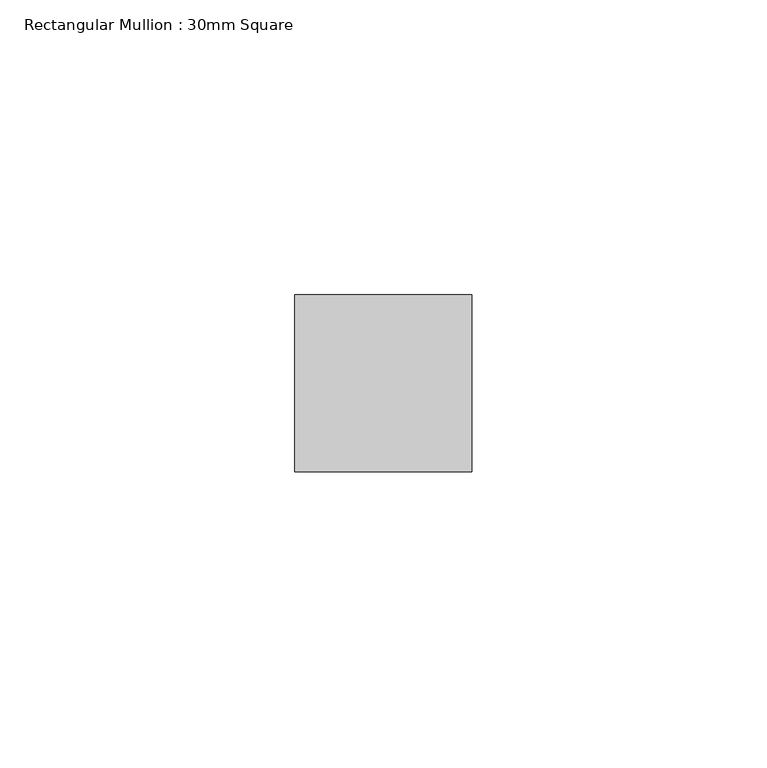
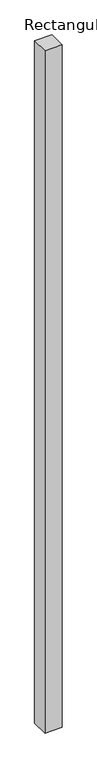
"""IFC4 building model written with IfcOpenShell, lengths in millimetres: member geometry, Rectangular Mullion : 30mm Square."""

from ifc_helpers import new_model, si_unit, frame, origin, place, context, project, spatial, polyline, outline, extrude, source, transform, mapped, element, save


def rectangular_mullion_30mm_square_7d0e1db8(model_context):
    return source(origin(), model_context, "Body", "SweptSolid", [
        extrude(outline(polyline([(15.0, 15.0), (15.0, -15.0), (-15.0, -15.0), (-15.0, 15.0), (15.0, 15.0)])), frame((0.0, 0.0, -1237.5), z_axis=(0.0, 0.0, 1.0), x_axis=(1.0, 0.0, 0.0)), (0.0, 0.0, 1.0), 1237.5),
    ])


if __name__ == "__main__":
    model = new_model("IFC4")
    model_context = context("Model", 3, world=origin())
    ifc_project = project(units=[si_unit("LENGTHUNIT", "METRE", prefix="MILLI")], contexts=[model_context])
    site = spatial("IfcSite", under=ifc_project)
    building = spatial("IfcBuilding", under=site)
    placement = place(None, origin())
    rectangular_mullion_30mm_square_shape = rectangular_mullion_30mm_square_7d0e1db8(model_context)
    element("IfcMember", 1, ObjectType="Rectangular Mullion : 30mm Square", at=placement, inside=building, context=model_context, shape_type="MappedRepresentation", body=[
        mapped(rectangular_mullion_30mm_square_shape, transform((0.0, 0.0, 0.0), x_axis=(1.0, 0.0, 0.0), y_axis=(0.0, 1.0, 0.0), z_axis=(0.0, 0.0, 1.0))),
    ])
    save(model, "model.ifc")

# Revit data of these elements
# Type "Rectangular Mullion : 30mm Square"
#   built-in parameter 1007304 = 0.0984252 (stored number, unit not read)
#   built-in parameter 1007301 = 0.0492126 (stored number, unit not read)
#   built-in parameter 1007300 = 0.0492126 (stored number, unit not read)
# Element 1 (IfcMember, "Rectangular Mullion : 30mm Square")
#   Materials on its faces: "Aluminum"
# Materials
#   "Aluminum": class "Metal", colour RGB 244 244 244, transparency 0, Description = "Aluminum 6061", Cost = 0
